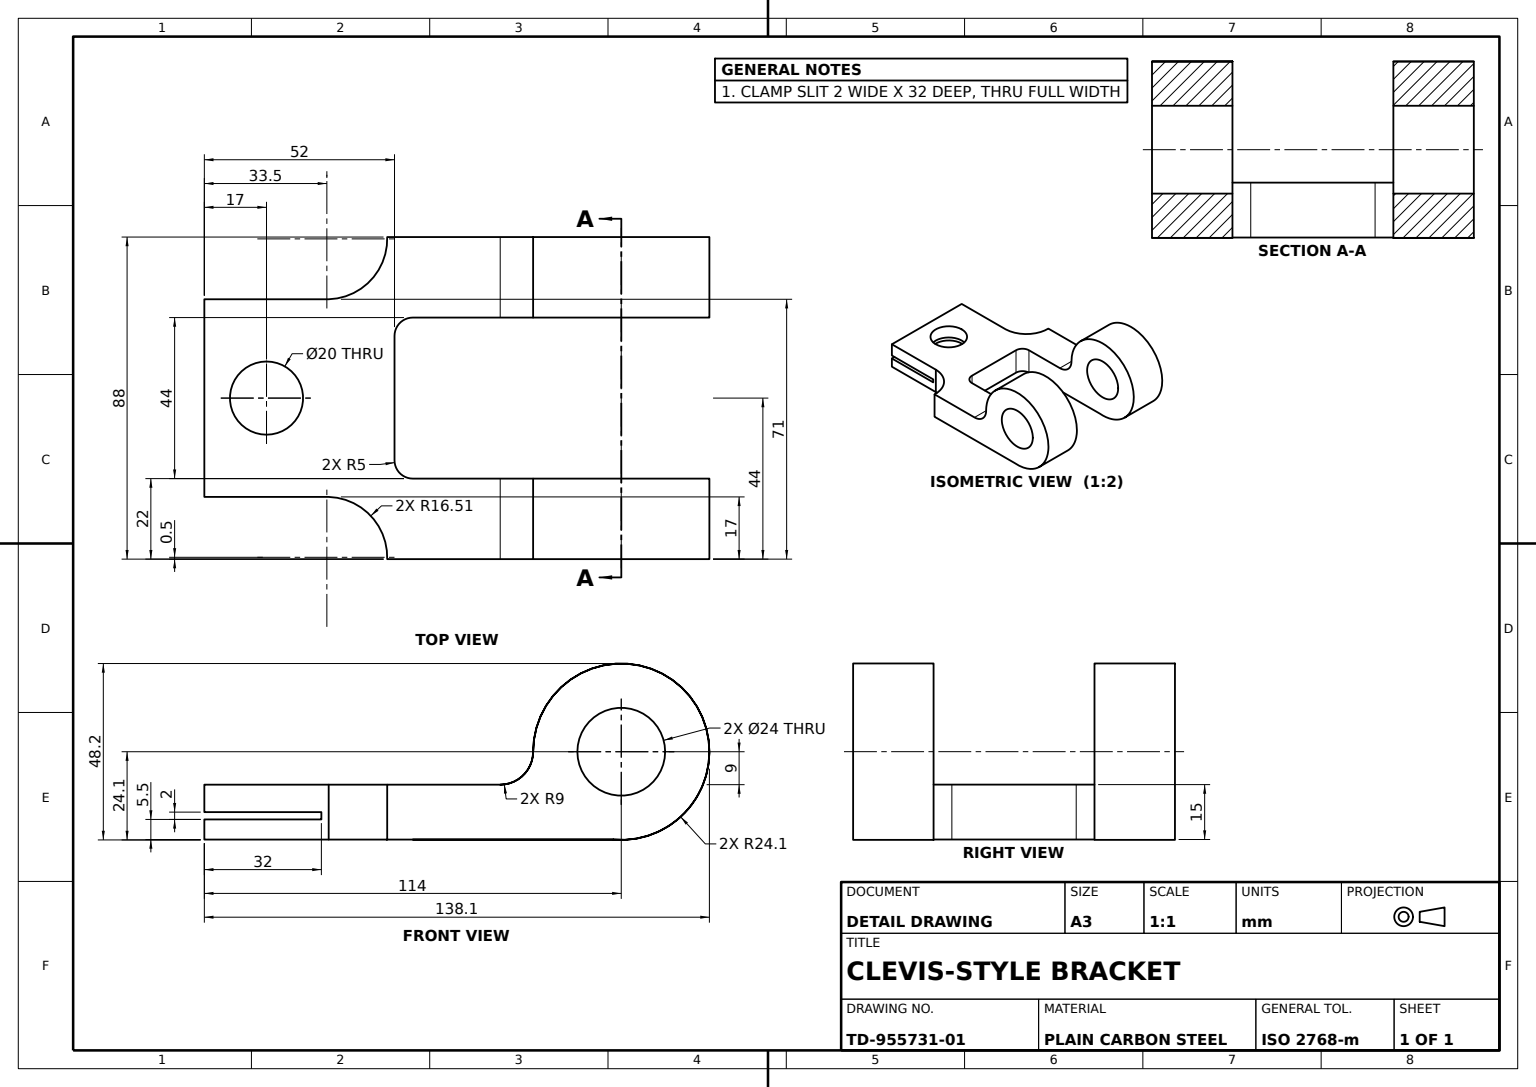
from build123d import *

# Parameters (mm, degrees)
BASE_PLATE_SKETCH_W               = 114
BASE_PLATE_SKETCH_H               = 88
BASE_PLATE_114X88X15_DEPTH        = 15
FORK_EYE_A_SKETCH_R               = 24.1
FORK_EYE_A_48_2_DEPTH             = 22
FORK_START                        = -22
FORK_EYE_B_SKETCH_R               = 24.1
FORK_EYE_B_48_2_DEPTH             = 22
EYE_BORE_SKETCH_R                 = 12
EYE_BORE_24_DEPTH                 = 129.976044287
FORK_FILLET_R9_R                  = 9
FORK_GAP_PROFILE_SKETCH_R         = 10
FORK_GAP_AND_CLAMP_HOLE_CUT_DEPTH = 99.024588752
CLAMP_SLIT_2MM_DEPTH              = 119.033130942
CLAMP_SLIT_2MM_DEPTH_BACK         = 119.033130942
CLAMP_SLIT_SKETCH_W               = 32
CLAMP_SLIT_SKETCH_H               = 2


with BuildPart() as part:
    # Base Plate Sketch → Base Plate 114x88x15 (new body)
    with BuildSketch(Plane(origin=(0, 0, 0), x_dir=(1, 0, 0), z_dir=(0, 1, 0))):
        Rectangle(BASE_PLATE_SKETCH_W, BASE_PLATE_SKETCH_H)
    extrude(amount=BASE_PLATE_114X88X15_DEPTH)

    # Fork Eye A Sketch → Fork Eye A Ø48.2 (add)
    with BuildSketch(Plane.XY.offset(44)):
        with Locations((57, 24)):
            Circle(FORK_EYE_A_SKETCH_R)
    extrude(amount=-FORK_EYE_A_48_2_DEPTH)

    # Fork Eye B Sketch → Fork Eye B Ø48.2 (add)
    with BuildSketch(Plane(origin=(0, 0, -44), x_dir=(-1, 0, 0), z_dir=(0, 0, -1)).offset(FORK_START)):
        with Locations((-57, 24)):
            Circle(FORK_EYE_B_SKETCH_R)
    extrude(amount=FORK_EYE_B_48_2_DEPTH)

    # Eye Bore Sketch → Eye Bore Ø24 (cut, through all)
    with BuildSketch(Plane(origin=(0, 0, -44), x_dir=(-1, 0, 0), z_dir=(0, 0, -1))):
        with Locations((-57, 24)):
            Circle(EYE_BORE_SKETCH_R)
    extrude(amount=-EYE_BORE_24_DEPTH, mode=Mode.SUBTRACT)

    # Fork Fillet R9
    fork_fillet_r9_edges = [part.edges().sort_by_distance(p)[0] for p in [
        (34.643569158, 15, 33),
        (34.643569158, 15, -33),
    ]]
    fillet(fork_fillet_r9_edges, radius=FORK_FILLET_R9_R)

    # Fork Gap Profile Sketch → Fork Gap and Clamp Hole Cut (cut, through all)
    with BuildSketch(Plane(origin=(0, 15, 0), x_dir=(1, 0, 0), z_dir=(0, 1, 0))):
        with Locations(Location((-40, 0, 0), (0, 0, 270))):
            Circle(FORK_GAP_PROFILE_SKETCH_R)
        with BuildLine():
            Line((57, 22), (0, 22))
            ThreePointArc((0, 22), (-3.535533906, 20.535533906), (-5, 17))
            Line((-5, 17), (-5, -17))
            ThreePointArc((-5, -17), (-3.535533906, -20.535533906), (0, -22))
            Line((0, -22), (57, -22))
            Line((57, -22), (57, 22))
        make_face()
        with BuildLine():
            Line((-57, 44), (-7, 44))
            ThreePointArc((-7, 44), (-11.47918472, 32.186291501), (-23, 27))
            Line((-23, 27), (-57, 27))
            Line((-57, 27), (-57, 44))
        make_face()
        with BuildLine():
            Line((-57, -44), (-7, -44))
            ThreePointArc((-7, -44), (-11.47918472, -32.186291501), (-23, -27))
            Line((-23, -27), (-57, -27))
            Line((-57, -27), (-57, -44))
        make_face()
    extrude(amount=-FORK_GAP_AND_CLAMP_HOLE_CUT_DEPTH, mode=Mode.SUBTRACT)

    # Clamp Slit Sketch → Clamp Slit 2mm (cut, two sides: drawn at the far end of the back side and taken through both)
    with BuildSketch(Plane(origin=(0, 0, -27), x_dir=(-1, 0, 0), z_dir=(0, 0, -1)).offset(-CLAMP_SLIT_2MM_DEPTH_BACK)):
        with Locations((41, 6.5)):
            Rectangle(CLAMP_SLIT_SKETCH_W, CLAMP_SLIT_SKETCH_H)
    extrude(amount=CLAMP_SLIT_2MM_DEPTH + CLAMP_SLIT_2MM_DEPTH_BACK, mode=Mode.SUBTRACT)


solid = part.part
